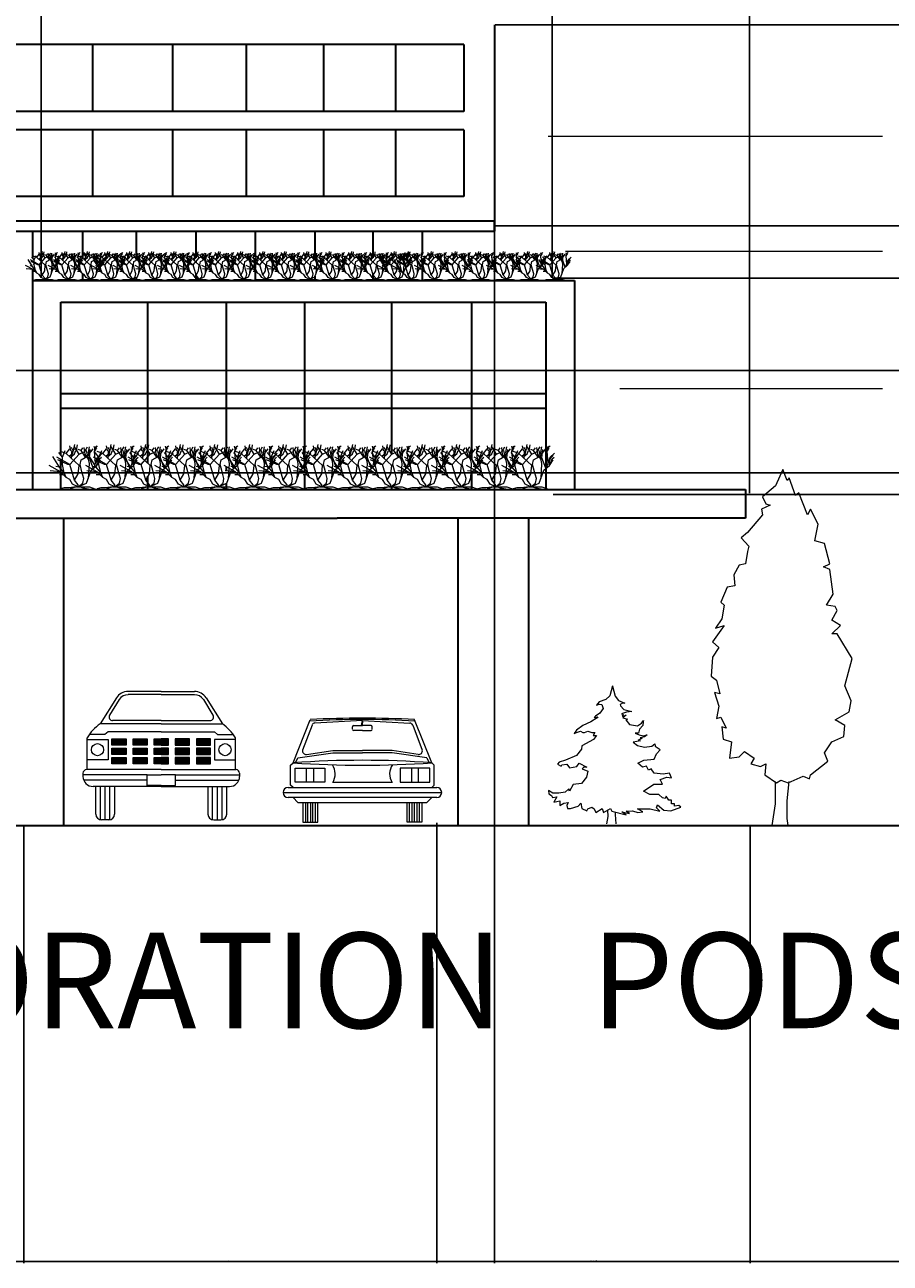
# Model space of a CAD drawing. Units: inches. Extents: x -160 to 434, y -145 to 103.
# Tile 5 of 7: x 176 to 262, y -145 to -22. Entities that reach past the tile are written whole.
import ezdxf

# ---------------------------------------------------------------- set-up
doc = ezdxf.new("R2010")
doc.units = ezdxf.units.IN
doc.header["$MEASUREMENT"] = 0
for name, color, linetype, lineweight in [('A-ANNO-DIMS', 2, 'Continuous', 18), ('A-ANNO-SYMB', 2, 'Continuous', 13), ('A-ANNO-TEXT', 3, 'Continuous', 18), ('A-ELEV', 7, 'Continuous', 35), ('A-ENTO-VEHC', 8, 'Continuous', 13), ('L-PLNT', 3, 'Continuous', 13)]:
    doc.layers.add(name, color=color, linetype=linetype, lineweight=lineweight)
doc.styles.get("Standard").update_dxf_attribs({"font": 'arial.ttf'})
doc.dimstyles.get("Standard").update_dxf_attribs({"dimtxt": 0.18, "dimasz": 0.18, "dimexe": 0.18, "dimexo": 0.0625, "dimgap": 0.09, "dimtad": 0, "dimtih": 1, "dimtoh": 1, "dimdec": 4, "dimzin": 0, "dimdsep": 46, "dimtxsty": 'Standard', "dimcen": 0.09, "dimadec": 0, "dimazin": 0, "dimtfac": 1, "dimtdec": 4, "dimtofl": 0, "dimtmove": 0, "dimatfit": 3, "dimfxl": 1, "dimtolj": 1, "dimtzin": 0, "dimarcsym": 0})

# ---------------------------------------------------------------- blocks, each defined once
blk = doc.blocks.new('*U2')
blk.add_lwpolyline([(-2.754, 191.699), (-6.78, 182.851), (-13.682, 176.953), (-11.956, 173.266), (-9.656, 172.529), (-14.257, 170.317), (-13.682, 167.368), (-21.733, 157.783), (-25.184, 154.834), (-21.158, 150.41), (-21.733, 147.461), (-22.884, 140.825), (-26.334, 140.087), (-29.21, 134.926), (-28.635, 129.028), (-32.661, 128.291), (-36.111, 120.18), (-34.386, 118.706), (-35.536, 111.333), (-38.987, 106.171), (-34.386, 107.646), (-40.712, 98.798), (-37.261, 95.849), (-40.712, 90.688), (-41.287, 80.366), (-38.412, 78.154), (-36.686, 70.781), (-39.562, 71.518), (-37.261, 64.145), (-38.412, 57.509), (-36.111, 58.247), (-33.236, 52.348), (-35.536, 53.086), (-34.961, 46.45), (-30.36, 44.975), (-31.51, 36.128), (-26.334, 36.865), (-23.459, 39.814), (-18.283, 36.128), (-20.008, 33.178), (-14.832, 31.704), (-11.956, 33.178), (-12.531, 27.28), (-6.205, 22.856), (-3.905, 24.331), (0.121, 22.856), (8.173, 26.543), (11.624, 25.068), (12.199, 27.28), (21.4, 34.653), (19.675, 39.077), (23.701, 44.975), (30.027, 47.924), (30.602, 53.823), (25.426, 56.772), (32.903, 61.196), (34.053, 67.094), (30.602, 75.205), (34.628, 89.951), (26.576, 103.222), (23.701, 103.222), (28.302, 107.646), (23.701, 110.595), (26.576, 115.756), (25.426, 117.968), (20.825, 118.706), (24.276, 124.604), (22.551, 137.876), (19.1, 139.35), (22.551, 140.825), (19.675, 151.884), (14.499, 153.359), (16.224, 162.207), (12.199, 170.317), (10.473, 167.368), (5.872, 179.165), (4.147, 177.69), (0.696, 187.275), (-0.454, 185.8)], close=True)
for points in [[(-6.813, 23.669), (-6.813, 11.669), (-8.627, 0)], [(0.387, 23.669), (-0.576, 13.271), (-0.576, 3.686), (0, 0)]]:
    blk.add_lwpolyline(points)
blk = doc.blocks.new('*U10')
for p, q in [((0, 69.27), (-17.87, 69.27)), ((0, 67.49), (-17.87, 67.49)), ((0, 69.27), (17.87, 69.27)), ((0, 67.49), (17.87, 67.49)), ((-24.18, 65.77), (-32.91, 51.76)), ((-22.67, 64.82), (-27.86, 56.49)), ((22.67, 64.82), (27.86, 56.49)), ((24.18, 65.77), (32.91, 51.76)), ((0, 53.54), (-26.22, 53.54)), ((0, 53.54), (26.22, 53.54)), ((0, 51.76), (-32.91, 51.76)), ((-28.59, 47.44), (-30.37, 45.96)), ((0, 47.44), (-28.59, 47.44)), ((0, 51.76), (32.91, 51.76)), ((0, 47.44), (28.59, 47.44)), ((28.59, 47.44), (30.37, 45.96)), ((-40.01, 27.08), (-40.01, 44.29)), ((-40.01, 43.31), (-28.69, 43.31)), ((-30.37, 45.96), (-38.87, 45.96)), ((-28.69, 43.31), (-28.69, 32.39)), ((-26.57, 40.26), (-26.57, 43.7)), ((-26.57, 43.7), (-18.89, 43.7)), ((-18.89, 40.26), (-26.57, 40.26)), ((-18.89, 43.7), (-18.89, 40.26)), ((-15.2, 43.7), (-7.53, 43.7)), ((-15.2, 40.26), (-15.2, 43.7)), ((-7.53, 40.26), (-15.2, 40.26)), ((-7.53, 43.7), (-7.53, 40.26)), ((-3.84, 40.26), (-3.84, 43.7)), ((-3.84, 43.7), (0, 43.7)), ((0, 40.26), (-3.84, 40.26)), ((3.84, 43.7), (0, 43.7)), ((0, 40.26), (3.84, 40.26)), ((3.84, 40.26), (3.84, 43.7)), ((7.53, 43.7), (7.53, 40.26)), ((15.2, 43.7), (7.53, 43.7)), ((7.53, 40.26), (15.2, 40.26)), ((15.2, 40.26), (15.2, 43.7)), ((26.57, 43.7), (18.89, 43.7)), ((18.89, 43.7), (18.89, 40.26)), ((18.89, 40.26), (26.57, 40.26)), ((26.57, 40.26), (26.57, 43.7)), ((28.69, 43.31), (28.69, 32.39)), ((40.01, 43.31), (28.69, 43.31)), ((30.37, 45.96), (38.87, 45.96)), ((40.01, 27.08), (40.01, 44.29)), ((-26.57, 35.24), (-26.57, 38.69)), ((-26.57, 38.69), (-18.89, 38.69)), ((-18.89, 35.24), (-26.57, 35.24)), ((-26.57, 30.23), (-26.57, 33.67)), ((-26.57, 33.67), (-18.89, 33.67)), ((-18.89, 38.69), (-18.89, 35.24)), ((-18.89, 33.67), (-18.89, 30.23)), ((-15.2, 38.69), (-7.53, 38.69)), ((-15.2, 35.24), (-15.2, 38.69)), ((-7.53, 35.24), (-15.2, 35.24)), ((-15.2, 33.67), (-7.53, 33.67)), ((-15.2, 30.23), (-15.2, 33.67)), ((-7.53, 38.69), (-7.53, 35.24)), ((-7.53, 33.67), (-7.53, 30.23)), ((-3.84, 35.24), (-3.84, 38.69)), ((-3.84, 38.69), (0, 38.69)), ((0, 35.24), (-3.84, 35.24)), ((-3.84, 30.23), (-3.84, 33.67)), ((-3.84, 33.67), (0, 33.67)), ((3.84, 38.69), (0, 38.69)), ((0, 35.24), (3.84, 35.24)), ((3.84, 33.67), (0, 33.67)), ((3.84, 35.24), (3.84, 38.69)), ((3.84, 30.23), (3.84, 33.67)), ((7.53, 38.69), (7.53, 35.24)), ((15.2, 38.69), (7.53, 38.69)), ((7.53, 35.24), (15.2, 35.24)), ((7.53, 33.67), (7.53, 30.23)), ((15.2, 33.67), (7.53, 33.67)), ((15.2, 35.24), (15.2, 38.69)), ((15.2, 30.23), (15.2, 33.67)), ((26.57, 38.69), (18.89, 38.69)), ((18.89, 38.69), (18.89, 35.24)), ((18.89, 35.24), (26.57, 35.24)), ((26.57, 33.67), (18.89, 33.67)), ((18.89, 33.67), (18.89, 30.23)), ((26.57, 35.24), (26.57, 38.69)), ((26.57, 30.23), (26.57, 33.67)), ((0, 27.08), (-40.3, 27.08)), ((-28.69, 32.39), (-40.01, 32.39)), ((-18.89, 30.23), (-26.57, 30.23)), ((-7.53, 30.23), (-15.2, 30.23)), ((0, 30.23), (-3.84, 30.23)), ((0, 30.23), (3.84, 30.23)), ((0, 27.08), (40.3, 27.08)), ((7.53, 30.23), (15.2, 30.23)), ((18.89, 30.23), (26.57, 30.23)), ((28.69, 32.39), (40.01, 32.39)), ((-42.18, 25.2), (-42.18, 23.46)), ((-7.63, 24.32), (-42.18, 24.32)), ((-7.63, 21.37), (-41.76, 21.37)), ((-7.63, 18.62), (-7.63, 24.32)), ((-7.63, 24.32), (0, 24.32)), ((7.63, 24.32), (0, 24.32)), ((7.63, 24.32), (42.18, 24.32)), ((7.63, 18.62), (7.63, 24.32)), ((7.63, 21.37), (41.76, 21.37)), ((42.18, 25.2), (42.18, 23.46)), ((0, 18.03), (-36.75, 18.03)), ((-35.26, 3.13), (-35.26, 18.03)), ((-32.73, 0.06), (-32.73, 18.03)), ((-30.2, 0), (-30.2, 18.03)), ((-27.66, 0.06), (-27.66, 18.03)), ((-25.13, 18.03), (-25.13, 3.13)), ((0, 18.62), (-7.63, 18.62)), ((0, 18.62), (7.63, 18.62)), ((0, 18.03), (36.75, 18.03)), ((25.13, 18.03), (25.13, 3.13)), ((27.66, 0.06), (27.66, 18.03)), ((30.2, 0), (30.2, 18.03)), ((32.73, 0.06), (32.73, 18.03)), ((35.26, 3.13), (35.26, 18.03)), ((-28.26, 0), (-32.13, 0)), ((28.26, 0), (32.13, 0))]:
    blk.add_line(p, q)
for centre in [(-34.35, 37.85), (34.35, 37.85)]:
    blk.add_circle(centre, 3.27)
for centre, radius, start, end in [((-17.87, 61.83), 7.44, 90, 148.09213), ((-17.87, 61.83), 5.65, 90, 148.09213), ((17.87, 61.83), 7.44, 31.90786, 90), ((17.87, 61.83), 5.65, 31.90786, 90), ((-26.22, 55.47), 1.92, 148.09213, 270), ((26.22, 55.47), 1.92, 270, 31.90786), ((-18.03, 30.48), 25.96, 124.96933, 147.86524), ((18.03, 30.48), 25.96, 32.13477, 55.03066), ((-40.3, 25.2), 1.88, 90, 180.00001), ((40.3, 25.2), 1.88, 0, 90), ((-36.75, 23.46), 5.43, 180.00001, 270), ((36.75, 23.46), 5.43, 270, 0), ((-32.13, 3.13), 3.13, 180.00001, 270), ((-28.26, 3.13), 3.13, 270, 0), ((28.26, 3.13), 3.13, 180.00001, 270), ((32.13, 3.13), 3.13, 270, 0)]:
    blk.add_arc(centre, radius, start, end)
for points in [[(-18.89, 43.7), (-18.89, 40.26), (-26.57, 43.7), (-26.57, 40.26)], [(-7.53, 43.7), (-7.53, 40.26), (-15.2, 43.7), (-15.2, 40.26)], [(0, 43.7), (0, 40.26), (-3.84, 43.7), (-3.84, 40.26)], [(0, 43.7), (0, 40.26), (3.84, 43.7), (3.84, 40.26)], [(7.53, 43.7), (7.53, 40.26), (15.2, 43.7), (15.2, 40.26)], [(18.89, 43.7), (18.89, 40.26), (26.57, 43.7), (26.57, 40.26)], [(-18.89, 38.69), (-18.89, 35.24), (-26.57, 38.69), (-26.57, 35.24)], [(-18.89, 33.67), (-18.89, 30.23), (-26.57, 33.67), (-26.57, 30.23)], [(-7.53, 38.69), (-7.53, 35.24), (-15.2, 38.69), (-15.2, 35.24)], [(-7.53, 33.67), (-7.53, 30.23), (-15.2, 33.67), (-15.2, 30.23)], [(0, 38.69), (0, 35.24), (-3.84, 38.69), (-3.84, 35.24)], [(0, 33.67), (0, 30.23), (-3.84, 33.67), (-3.84, 30.23)], [(0, 38.69), (0, 35.24), (3.84, 38.69), (3.84, 35.24)], [(0, 33.67), (0, 30.23), (3.84, 33.67), (3.84, 30.23)], [(7.53, 38.69), (7.53, 35.24), (15.2, 38.69), (15.2, 35.24)], [(7.53, 33.67), (7.53, 30.23), (15.2, 33.67), (15.2, 30.23)], [(18.89, 38.69), (18.89, 35.24), (26.57, 38.69), (26.57, 35.24)], [(18.89, 33.67), (18.89, 30.23), (26.57, 33.67), (26.57, 30.23)]]:
    blk.add_solid(points)
blk = doc.blocks.new('*U11')
for p, q in [((-37.38, 32.04), (-28.11, 55.23)), ((-0.21, 54.74), (-0.67, 52.07)), ((0.21, 54.74), (-0.23, 52.08)), ((37.38, 32.04), (28.11, 55.23)), ((-36.05, 32.04), (-34.71, 34.71)), ((-34.71, 34.71), (-16.02, 37.38)), ((-16.02, 37.38), (0, 37.38)), ((16.02, 37.38), (0, 37.38)), ((34.71, 34.71), (16.02, 37.38)), ((34.71, 34.71), (36.05, 32.04)), ((-38.72, 30.71), (-37.38, 32.04)), ((-38.72, 20.03), (-38.72, 30.71)), ((38.72, 30.71), (37.38, 32.04)), ((38.72, 20.03), (38.72, 30.71)), ((-37.38, 18.69), (-38.72, 20.03)), ((16.02, 21.36), (-16.02, 21.36)), ((37.38, 18.69), (38.72, 20.03)), ((-42.72, 16.02), (42.72, 16.02)), ((-40.05, 18.69), (40.05, 18.69)), ((40.05, 13.35), (-40.05, 13.35)), ((-37.38, 13.35), (-34.71, 10.68)), ((34.71, 10.68), (37.38, 13.35)), ((-34.71, 10.68), (34.71, 10.68)), ((-32.04, 10.68), (-32.04, 0)), ((-30.71, 10.68), (-30.71, 0)), ((-29.37, 0), (-29.37, 10.68)), ((-28.04, 10.68), (-28.04, 0)), ((-26.7, 0), (-26.7, 10.68)), ((-25.37, 10.68), (-25.37, 0)), ((-24.03, 0), (-24.03, 10.68)), ((24.03, 0), (24.03, 10.68)), ((25.37, 0), (25.37, 10.68)), ((26.7, 10.68), (26.7, 0)), ((28.04, 0), (28.04, 10.68)), ((29.37, 10.68), (29.37, 0)), ((30.71, 0), (30.71, 10.68)), ((32.04, 10.68), (32.04, 0)), ((-32.04, 0), (-24.03, 0)), ((32.04, 0), (24.03, 0))]:
    blk.add_line(p, q)
for points in [[(0, 54.74), (-25.63, 53.46)], [(0.01, 54.74), (25.64, 53.45)], [(-27.12, 52.31), (-32.28, 38.89)], [(-5.34, 50.07), (-5.34, 51.4)], [(-4.67, 52.07), (0, 52.07)], [(0, 49.4), (-4.67, 49.4)], [(4.67, 52.07), (0, 52.07)], [(0, 49.4), (4.67, 49.4)], [(5.34, 50.07), (5.34, 51.4)], [(27.13, 52.3), (32.28, 38.88)], [(-30.06, 36.56), (-16.02, 38.72), (0, 38.72)], [(30.06, 36.54), (16.02, 38.71), (0, 38.72)]]:
    blk.add_lwpolyline(points)
for points in [[(-36.27, 29.17), (-20.26, 29.17), (-20.26, 21.57), (-36.27, 21.57)], [(-30.17, 29.17), (-26.37, 29.17), (-26.37, 21.57), (-30.17, 21.57)], [(36.27, 29.17), (20.26, 29.17), (20.26, 21.57), (36.27, 21.57)], [(30.17, 29.17), (26.37, 29.17), (26.37, 21.57), (30.17, 21.57)]]:
    blk.add_lwpolyline(points, close=True)
for centre, radius, start, end in [((0, -432), 487.32, 86.65721, 93.3419), ((0, -431.24), 487.32, 86.69396, 93.3033), ((-25.37, 51.59), 1.89, 97.4497, 154.9311), ((25.37, 51.57), 1.89, 25.04208, 82.52346), ((-4.67, 51.4), 0.668, 93.60832, 178.1081), ((-4.67, 50.07), 0.668, 184.4192, 266.4386), ((4.67, 51.4), 0.668, 1.89193, 86.39168), ((4.67, 50.07), 0.668, 273.5614, 355.5808), ((0, -490.66), 524.03, 85.90918, 94.09081), ((-30.43, 38.42), 1.89, 166.5724, 279.9572), ((30.43, 38.41), 1.89, 260.016, 13.40079), ((0, 554.74), 524.03, 265.90919, 274.09082), ((-23.36, 26.03), 8.7, 327.5288, 34.44428), ((23.36, 26.03), 8.7, 145.55569, 212.4712), ((-40.05, 16.02), 2.67, 90, 270), ((40.05, 16.02), 2.67, 270, 90)]:
    blk.add_arc(centre, radius, start, end)
blk = doc.blocks.new('*U5')
for p, q in [((-14.88, 18.24), (-17.76, 19.2)), ((-16.8, 16.32), (-15.36, 19.68)), ((-14.88, 18.24), (-12.96, 20.64)), ((-12.471, 19.775), (-12.898, 22.044)), ((-11.677, 19.071), (-12.471, 19.775)), ((-11.28, 19.619), (-12.104, 21.184)), ((-11.921, 18.836), (-10.64, 20.401)), ((-11.433, 18.289), (-10.457, 22.749)), ((-10.579, 18.054), (-9.846, 19.697)), ((-8.16, 17.76), (-10.56, 21.6)), ((-9.48, 19.775), (-8.992, 22.592)), ((-7.2, 19.68), (-8.64, 20.16)), ((-8.16, 17.76), (-5.28, 19.2)), ((-7.2, 19.68), (-6.24, 21.12)), ((-4.8, 16.32), (-7.2, 19.68)), ((-5.086, 17.741), (-5.513, 21.34)), ((-5.28, 19.2), (-3.84, 21.6)), ((-2.88, 12.96), (-4.32, 19.68)), ((-3.84, 16.8), (-0.96, 20.64)), ((-3.377, 18.602), (-2.888, 21.575)), ((-2.88, 15.84), (-2.4, 20.16)), ((-0.508, 21.888), (-0.081, 20.558)), ((-0.203, 19.149), (0.102, 21.34)), ((-0.142, 19.384), (0.59, 20.401)), ((-0.02, 20.01), (0.896, 21.105)), ((0.041, 20.714), (1.384, 22.044)), ((0.102, 21.34), (0.835, 21.888)), ((-18.24, 11.04), (-21.755, 16.655)), ((-12.96, 12.48), (-19.68, 16.32)), ((-13.92, 12.48), (-19.2, 14.88)), ((-16.8, 16.32), (-18.72, 18.72)), ((-16.8, 12.48), (-17.76, 12.96)), ((-16.8, 12.48), (-16.8, 16.32)), ((-8.16, 12), (-14.88, 18.24)), ((-13.325, 16.724), (-11.433, 18.289)), ((-12.96, 12.48), (-8.16, 17.76)), ((-12.043, 15.628), (-11.921, 18.836)), ((-11.982, 16.802), (-10.579, 18.054)), ((-7.68, 12.48), (-7.2, 14.88)), ((-7.2, 14.88), (-3.84, 16.8)), ((-3.377, 15.315), (-5.086, 17.819)), ((-2.766, 16.802), (-3.377, 18.602)), ((-3.36, 5.28), (-2.88, 12.96)), ((-0.96, 10.56), (-2.88, 15.84)), ((-0.48, 10.8), (0.346, 13.203)), ((0.346, 13.203), (-0.203, 19.149)), ((0.346, 13.203), (1.323, 16.254)), ((0.96, 12), (1.44, 15.36)), ((0.96, 12), (2.88, 14.88)), ((1.323, 16.254), (3.642, 18.289)), ((1.44, 15.36), (2.88, 17.28)), ((1.92, 13.44), (2.4, 15.36)), ((2.4, 15.36), (3.36, 16.32)), ((-17.76, 8.64), (-23.663, 11.961)), ((-17.76, 8.64), (-23.128, 9.222)), ((-18.24, 11.04), (-20.16, 11.52)), ((-15.84, 8.16), (-18.24, 11.04)), ((-16.32, 7.2), (-18.24, 7.2)), ((-14.88, 5.76), (-17.76, 8.64)), ((-15.84, 8.16), (-16.8, 12.48)), ((-14.88, 5.76), (-15.84, 8.16)), ((-12.96, 12.48), (-13.92, 12.48)), ((-10.56, 4.32), (-12.96, 12.48)), ((-10.56, 4.32), (-8.64, 7.68)), ((-8.64, 7.68), (-8.16, 12)), ((-6.72, 8.64), (-7.68, 12.48)), ((-5.76, 5.28), (-6.72, 8.64)), ((-4.32, 2.88), (-1.92, 9.6)), ((-1.92, 9.6), (0.96, 12)), ((-15.84, 0.48), (-17.76, 0)), ((-13.44, 0.48), (-15.84, 0.48)), ((-12.96, 4.8), (-14.88, 5.76)), ((-9.6, 0.96), (-13.44, 0.48)), ((-11.52, 2.4), (-12.96, 4.8)), ((-9.6, 0.96), (-12.96, 0)), ((-8.64, 0.96), (-11.52, 2.4)), ((-8.64, 1.92), (-10.56, 4.32)), ((-9.6, 0.96), (-7.68, 0.96)), ((-8.64, 0.96), (-4.32, 2.88)), ((-8.64, 0.96), (-6.24, 2.88)), ((-8.64, 0.96), (-8.64, 1.92)), ((-8.64, 0.96), (-2.88, 0.96)), ((-7.68, 0.96), (-6.24, 0.48)), ((-6.24, 2.88), (-5.76, 5.28)), ((-6.24, 0.48), (-3.36, 0)), ((-2.88, 0.96), (0, 0))]:
    blk.add_line(p, q)
blk = doc.blocks.new('*U7')
for p, q in [((-8.263, 7.598), (-8.747, 14.105)), ((-9.75, 0), (-8.263, 7.598)), ((-0.771, 9.56), (-0.69, 11.833)), ((0, 0), (-0.771, 9.56))]:
    blk.add_line(p, q)
for points in [[(-3.9, 142.35), (-6.596, 132.037), (-10.801, 128.443), (-17.81, 126.047), (-20.614, 122.452), (-17.81, 123.65), (-15.007, 123.051), (-13.605, 118.858), (-16.876, 114.065), (-21.549, 111.07), (-22.951, 109.872), (-19.212, 110.471), (-19.68, 109.273), (-26.222, 105.079), (-34.633, 101.485), (-41.175, 96.693), (-43.511, 93.098), (-41.175, 94.296), (-36.969, 95.494), (-34.633, 94.296), (-32.764, 94.296), (-29.493, 95.494)], [(-3.759, 141.97), (-1.074, 131.643), (2.437, 127.141), (8.84, 124.493), (6.568, 124.493), (4.09, 123.169), (4.296, 121.846), (7.807, 117.874), (16.069, 116.02), (10.492, 115.226), (5.535, 113.372), (6.981, 112.843), (5.948, 110.989), (10.286, 112.048), (6.775, 109.401), (11.732, 108.077), (9.873, 107.282), (13.797, 102.516), (21.852, 101.192), (25.983, 103.84), (28.048, 106.488), (27.842, 105.164), (27.429, 101.457), (24.124, 97.75), (23.091, 93.513), (19.58, 93.513), (23.505, 91.66), (28.255, 90.866), (31.973, 91.925), (29.081, 89.806), (24.537, 88.747), (26.809, 88.218), (22.472, 86.099), (24.95, 85.57), (17.308, 84.246), (21.852, 80.804), (29.081, 79.215), (36.723, 80.009), (39.821, 82.392), (40.028, 80.009), (45.398, 76.567)], [(-29.25, 95.55), (-25.287, 94.296), (-22.016, 94.296), (-23.885, 91.301), (-20.614, 91.301), (-23.418, 87.108), (-35.567, 80.518), (-36.035, 76.924), (-41.175, 70.334), (-52.389, 65.542), (-58.931, 63.744), (-60.8, 61.348), (-57.062, 59.551), (-56.128, 60.749), (-50.987, 61.348), (-48.184, 57.754), (-40.707, 58.952), (-38.371, 62.546), (-30.427, 58.353), (-33.698, 58.353), (-35.1, 56.556), (-29.493, 54.159), (-30.894, 48.169), (-36.035, 41.579), (-44.446, 40.381), (-48.184, 33.791), (-49.118, 36.188), (-52.857, 32.593), (-59.399, 31.395), (-65.473, 31.395), (-70.146, 34.39), (-69.679, 30.796), (-66.875, 28.999), (-65.941, 27.202), (-61.268, 27.801), (-64.539, 22.409), (-58.464, 23.607), (-58.464, 18.815), (-54.258, 21.211), (-49.586, 21.81), (-50.987, 18.815), (-50.52, 15.82), (-47.249, 15.82), (-39.306, 18.216), (-36.502, 21.211), (-35.567, 15.82), (-30.427, 13.423), (-29.493, 15.221), (-25.287, 17.018), (-22.951, 15.221), (-21.081, 11.626), (-14.539, 15.82), (-13.138, 11.626), (-6.128, 15.82), (-4.726, 12.824), (10.226, 9.23), (5.554, 12.225), (13.497, 10.428), (10.226, 12.824), (16.768, 13.423), (22.376, 11.626), (27.516, 12.225), (21.909, 15.221), (34.993, 15.221), (44.806, 12.824), (41.535, 16.419), (42.469, 19.414), (49.011, 14.023), (56.487, 13.423), (66.768, 17.018), (64.431, 18.815), (60.226, 18.216), (60.226, 20.612), (56.955, 20.612), (56.955, 24.206), (54.151, 24.206), (51.348, 28.4), (50.413, 26.004), (47.609, 26.603), (43.871, 30.197), (38.731, 30.197), (34.525, 30.197), (27.983, 33.791), (38.731, 40.98), (47.609, 40.98), (45.273, 45.773), (52.282, 48.169), (56.955, 47.57), (55.086, 52.362), (48.544, 51.164), (39.198, 52.362), (35.927, 56.556), (33.123, 55.357), (31.254, 59.551), (27.049, 58.353), (22.376, 62.546), (28.451, 65.542), (39.198, 66.74), (41.535, 72.131), (45.273, 76.325)]]:
    blk.add_lwpolyline(points)
blk = doc.blocks.new('*D12')
at = {"layer": 'A-ANNO-DIMS', "color": 0, "lineweight": -2, "transparency": 16777216}
for p, q in [((-84.07, -101.41), (-84.07, -144.81)), ((403.75, -101.41), (403.75, -144.81)), ((-83.89, -144.63), (159.44, -144.63)), ((403.57, -144.63), (160.24, -144.63))]:
    blk.add_line(p, q, dxfattribs=at)
at = {"layer": 'A-ANNO-DIMS', "color": 0, "transparency": 16777216}
for points in [[(-83.89, -144.6), (-83.89, -144.66), (-84.07, -144.63)], [(403.57, -144.6), (403.57, -144.66), (403.75, -144.63)]]:
    blk.add_solid(points, dxfattribs=at)
at = {"layer": 'Defpoints', "color": 0, "transparency": 16777216}
for p in [(-84.07, -101.35), (403.75, -101.35), (403.75, -144.63)]:
    blk.add_point(p, dxfattribs=at)
at = {"layer": 'A-ANNO-DIMS', "color": 0, "transparency": 16777216, "insert": (159.84, -144.63), "char_height": 0.18, "attachment_point": 5}
blk.add_mtext('\\A1;487.8', dxfattribs=at)
blk = doc.blocks.new('*D22')
at = {"layer": 'A-ANNO-DIMS', "color": 0, "lineweight": -2, "transparency": 16777216}
for p, q in [((175.81, -101.41), (175.81, -144.81)), ((216.81, -101.09), (216.81, -144.81)), ((175.99, -144.63), (195.91, -144.63)), ((216.63, -144.63), (196.71, -144.63))]:
    blk.add_line(p, q, dxfattribs=at)
at = {"layer": 'A-ANNO-DIMS', "color": 0, "transparency": 16777216}
for points in [[(175.99, -144.6), (175.99, -144.66), (175.81, -144.63)], [(216.63, -144.6), (216.63, -144.66), (216.81, -144.63)]]:
    blk.add_solid(points, dxfattribs=at)
at = {"layer": 'Defpoints', "color": 0, "transparency": 16777216}
for p in [(175.81, -101.35), (216.81, -101.02), (216.81, -144.63)]:
    blk.add_point(p, dxfattribs=at)
at = {"layer": 'A-ANNO-DIMS', "color": 0, "transparency": 16777216, "insert": (196.31, -144.63), "char_height": 0.18, "attachment_point": 5}
blk.add_mtext('\\A1;40.99', dxfattribs=at)
blk = doc.blocks.new('*D23')
at = {"layer": 'A-ANNO-DIMS', "color": 0, "lineweight": -2, "transparency": 16777216}
for p, q in [((216.81, -101.09), (216.81, -144.81)), ((247.94, -101.38), (247.94, -144.81)), ((216.99, -144.63), (231.91, -144.63)), ((247.76, -144.63), (232.84, -144.63))]:
    blk.add_line(p, q, dxfattribs=at)
at = {"layer": 'A-ANNO-DIMS', "color": 0, "transparency": 16777216}
for points in [[(216.99, -144.6), (216.99, -144.66), (216.81, -144.63)], [(247.76, -144.6), (247.76, -144.66), (247.94, -144.63)]]:
    blk.add_solid(points, dxfattribs=at)
at = {"layer": 'Defpoints', "color": 0, "transparency": 16777216}
for p in [(216.81, -101.02), (247.94, -101.32), (247.94, -144.63)]:
    blk.add_point(p, dxfattribs=at)
at = {"layer": 'A-ANNO-DIMS', "color": 0, "transparency": 16777216, "insert": (232.37, -144.63), "char_height": 0.18, "attachment_point": 5}
blk.add_mtext('\\A1;31.135', dxfattribs=at)
blk = doc.blocks.new('*D31')
at = {"layer": 'A-ANNO-DIMS', "color": 0, "lineweight": -2, "transparency": 16777216}
for p, q in [((107.33, 8.95), (433.98, 8.95)), ((433.8, 8.77), (433.8, -23.43)), ((433.8, -55.99), (433.8, -23.79)), ((107.33, -56.17), (433.98, -56.17))]:
    blk.add_line(p, q, dxfattribs=at)
at = {"layer": 'A-ANNO-DIMS', "color": 0, "transparency": 16777216}
for points in [[(433.77, 8.77), (433.83, 8.77), (433.8, 8.95)], [(433.77, -55.99), (433.83, -55.99), (433.8, -56.17)]]:
    blk.add_solid(points, dxfattribs=at)
at = {"layer": 'Defpoints', "color": 0, "transparency": 16777216}
for p in [(107.27, 8.95), (107.27, -56.17), (433.8, -56.17)]:
    blk.add_point(p, dxfattribs=at)
at = {"layer": 'A-ANNO-DIMS', "color": 0, "transparency": 16777216, "insert": (433.8, -23.61), "char_height": 0.18, "attachment_point": 5}
blk.add_mtext('\\A1;65.11', dxfattribs=at)
blk = doc.blocks.new('*D32')
at = {"layer": 'A-ANNO-DIMS', "color": 0, "lineweight": -2, "transparency": 16777216}
for p, q in [((107.33, -56.17), (433.98, -56.17)), ((433.8, -56.35), (433.8, -61.07)), ((433.8, -66.15), (433.8, -61.43)), ((106.73, -66.33), (433.98, -66.33))]:
    blk.add_line(p, q, dxfattribs=at)
at = {"layer": 'A-ANNO-DIMS', "color": 0, "transparency": 16777216}
for points in [[(433.77, -56.35), (433.83, -56.35), (433.8, -56.17)], [(433.77, -66.15), (433.83, -66.15), (433.8, -66.33)]]:
    blk.add_solid(points, dxfattribs=at)
at = {"layer": 'Defpoints', "color": 0, "transparency": 16777216}
for p in [(107.27, -56.17), (106.67, -66.33), (433.8, -66.33)]:
    blk.add_point(p, dxfattribs=at)
at = {"layer": 'A-ANNO-DIMS', "color": 0, "transparency": 16777216, "insert": (433.8, -61.25), "char_height": 0.18, "attachment_point": 5}
blk.add_mtext('\\A1;10.165', dxfattribs=at)
blk = doc.blocks.new('*D41')
at = {"layer": 'A-ANNO-DIMS', "color": 0, "lineweight": -2, "transparency": 16777216}
for p, q in [((124.65, -41.4), (124.65, -144.81)), ((222.55, -41.85), (222.55, -144.81)), ((124.83, -144.63), (173.28, -144.63)), ((222.37, -144.63), (173.93, -144.63))]:
    blk.add_line(p, q, dxfattribs=at)
at = {"layer": 'A-ANNO-DIMS', "color": 0, "transparency": 16777216}
for points in [[(124.83, -144.6), (124.83, -144.66), (124.65, -144.63)], [(222.37, -144.6), (222.37, -144.66), (222.55, -144.63)]]:
    blk.add_solid(points, dxfattribs=at)
at = {"layer": 'Defpoints', "color": 0, "transparency": 16777216}
for p in [(124.65, -41.34), (222.55, -41.79), (222.55, -144.63)]:
    blk.add_point(p, dxfattribs=at)
at = {"layer": 'A-ANNO-DIMS', "color": 0, "transparency": 16777216, "insert": (173.6, -144.63), "char_height": 0.18, "attachment_point": 5}
blk.add_mtext('\\A1;97.9', dxfattribs=at)
blk = doc.blocks.new('*D42')
at = {"layer": 'A-ANNO-DIMS', "color": 0, "lineweight": -2, "transparency": 16777216}
for p, q in [((222.59, -21.84), (433.98, -21.84)), ((433.8, -22.02), (433.8, -31.63)), ((433.8, -41.61), (433.8, -31.99)), ((222.62, -41.79), (433.98, -41.79))]:
    blk.add_line(p, q, dxfattribs=at)
at = {"layer": 'A-ANNO-DIMS', "color": 0, "transparency": 16777216}
for points in [[(433.77, -22.02), (433.83, -22.02), (433.8, -21.84)], [(433.77, -41.61), (433.83, -41.61), (433.8, -41.79)]]:
    blk.add_solid(points, dxfattribs=at)
at = {"layer": 'Defpoints', "color": 0, "transparency": 16777216}
for p in [(222.53, -21.84), (222.55, -41.79), (433.8, -41.79)]:
    blk.add_point(p, dxfattribs=at)
at = {"layer": 'A-ANNO-DIMS', "color": 0, "transparency": 16777216, "insert": (433.8, -31.81), "char_height": 0.18, "attachment_point": 5}
blk.add_mtext('\\A1;19.946', dxfattribs=at)
blk = doc.blocks.new('*D43')
at = {"layer": 'A-ANNO-DIMS', "color": 0, "lineweight": -2, "transparency": 16777216}
for p, q in [((222.5, -5.64), (433.98, -5.64)), ((433.8, -5.82), (433.8, -13.56)), ((433.8, -21.66), (433.8, -13.92)), ((222.59, -21.84), (433.98, -21.84))]:
    blk.add_line(p, q, dxfattribs=at)
at = {"layer": 'A-ANNO-DIMS', "color": 0, "transparency": 16777216}
for points in [[(433.77, -5.82), (433.83, -5.82), (433.8, -5.64)], [(433.77, -21.66), (433.83, -21.66), (433.8, -21.84)]]:
    blk.add_solid(points, dxfattribs=at)
at = {"layer": 'Defpoints', "color": 0, "transparency": 16777216}
for p in [(222.44, -5.64), (222.53, -21.84), (433.8, -21.84)]:
    blk.add_point(p, dxfattribs=at)
at = {"layer": 'A-ANNO-DIMS', "color": 0, "transparency": 16777216, "insert": (433.8, -13.74), "char_height": 0.18, "attachment_point": 5}
blk.add_mtext('\\A1;16.204', dxfattribs=at)
blk = doc.blocks.new('*D44')
at = {"layer": 'A-ANNO-DIMS', "color": 0, "lineweight": -2, "transparency": 16777216}
for p, q in [((177.54, -46.95), (177.54, 102.5)), ((177.72, 102.32), (202.52, 102.32)), ((228.07, 102.32), (203.27, 102.32)), ((228.25, -46.95), (228.25, 102.5))]:
    blk.add_line(p, q, dxfattribs=at)
at = {"layer": 'A-ANNO-DIMS', "color": 0, "transparency": 16777216}
for points in [[(177.72, 102.35), (177.72, 102.29), (177.54, 102.32)], [(228.07, 102.35), (228.07, 102.29), (228.25, 102.32)]]:
    blk.add_solid(points, dxfattribs=at)
at = {"layer": 'Defpoints', "color": 0, "transparency": 16777216}
for p in [(228.25, 102.32), (177.54, -47.01), (228.25, -47.01)]:
    blk.add_point(p, dxfattribs=at)
at = {"layer": 'A-ANNO-DIMS', "color": 0, "transparency": 16777216, "insert": (202.89, 102.32), "char_height": 0.18, "attachment_point": 5}
blk.add_mtext('\\A1;50.71', dxfattribs=at)
blk = doc.blocks.new('*D45')
at = {"layer": 'A-ANNO-DIMS', "color": 0, "lineweight": -2, "transparency": 16777216}
for p, q in [((228.31, -47.01), (433.98, -47.01)), ((433.8, -47.19), (433.8, -57.57)), ((433.8, -68.3), (433.8, -57.93)), ((228.35, -68.48), (433.98, -68.48))]:
    blk.add_line(p, q, dxfattribs=at)
at = {"layer": 'A-ANNO-DIMS', "color": 0, "transparency": 16777216}
for points in [[(433.77, -47.19), (433.83, -47.19), (433.8, -47.01)], [(433.77, -68.3), (433.83, -68.3), (433.8, -68.48)]]:
    blk.add_solid(points, dxfattribs=at)
at = {"layer": 'Defpoints', "color": 0, "transparency": 16777216}
for p in [(228.25, -47.01), (228.29, -68.48), (433.8, -68.48)]:
    blk.add_point(p, dxfattribs=at)
at = {"layer": 'A-ANNO-DIMS', "color": 0, "transparency": 16777216, "insert": (433.8, -57.75), "char_height": 0.18, "attachment_point": 5}
blk.add_mtext('\\A1;21.473', dxfattribs=at)
blk = doc.blocks.new('*D46')
at = {"layer": 'A-ANNO-DIMS', "color": 0, "lineweight": -2, "transparency": 16777216}
for p, q in [((222.62, -41.79), (433.98, -41.79)), ((433.8, -41.97), (433.8, -54.95)), ((433.8, -68.3), (433.8, -55.32)), ((228.35, -68.48), (433.98, -68.48))]:
    blk.add_line(p, q, dxfattribs=at)
at = {"layer": 'A-ANNO-DIMS', "color": 0, "transparency": 16777216}
for points in [[(433.77, -41.97), (433.83, -41.97), (433.8, -41.79)], [(433.77, -68.3), (433.83, -68.3), (433.8, -68.48)]]:
    blk.add_solid(points, dxfattribs=at)
at = {"layer": 'Defpoints', "color": 0, "transparency": 16777216}
for p in [(222.55, -41.79), (228.29, -68.48), (433.8, -68.48)]:
    blk.add_point(p, dxfattribs=at)
at = {"layer": 'A-ANNO-DIMS', "color": 0, "transparency": 16777216, "insert": (433.8, -55.14), "char_height": 0.18, "attachment_point": 5}
blk.add_mtext('\\A1;26.7', dxfattribs=at)
blk = doc.blocks.new('*D48')
at = {"layer": 'A-ANNO-DIMS', "color": 0, "lineweight": -2, "transparency": 16777216}
for p, q in [((228.25, -46.95), (228.25, 102.5)), ((228.43, 102.32), (237.61, 102.32)), ((247.69, 102.32), (238.52, 102.32)), ((247.87, -68.35), (247.87, 102.5))]:
    blk.add_line(p, q, dxfattribs=at)
at = {"layer": 'A-ANNO-DIMS', "color": 0, "transparency": 16777216}
for points in [[(228.43, 102.35), (228.43, 102.29), (228.25, 102.32)], [(247.69, 102.35), (247.69, 102.29), (247.87, 102.32)]]:
    blk.add_solid(points, dxfattribs=at)
at = {"layer": 'Defpoints', "color": 0, "transparency": 16777216}
for p in [(247.87, 102.32), (228.25, -47.01), (247.87, -68.41)]:
    blk.add_point(p, dxfattribs=at)
at = {"layer": 'A-ANNO-DIMS', "color": 0, "transparency": 16777216, "insert": (238.06, 102.32), "char_height": 0.18, "attachment_point": 5}
blk.add_mtext('\\A1;19.626', dxfattribs=at)

msp = doc.modelspace()

# ---------------------------------------------------------------- linework, layer by layer
at = {"layer": 'A-ANNO-SYMB'}
for p, q in [((227.8844, -32.9114), (261.0586, -32.9114)), ((229.5882, -44.311), (261.0586, -44.311)), ((234.9964, -57.9615), (261.0586, -57.9615))]:
    msp.add_line(p, q, dxfattribs=at)
at = {"layer": 'A-ELEV'}
for p, q in [((222.5284, -21.8399), (222.5284, -41.3403)), ((219.5071, -23.7966), (137.8943, -23.7966)), ((182.6363, -23.7966), (182.6363, -30.4469)), ((190.5577, -23.7966), (190.5577, -30.4469)), ((197.8904, -23.7966), (197.8904, -30.4469)), ((205.5441, -23.7966), (205.5441, -30.4469)), ((212.7162, -23.7966), (212.7162, -30.4469)), ((219.5071, -23.7966), (219.5071, -30.4469)), ((219.5071, -30.4469), (137.8943, -30.4469)), ((219.5071, -32.2746), (137.8943, -32.2746)), ((182.6363, -32.2746), (182.6363, -38.9063)), ((190.5577, -32.2746), (190.5577, -38.9063)), ((197.8904, -32.2746), (197.8904, -38.9063)), ((205.5441, -32.2746), (205.5441, -38.9063)), ((212.7162, -32.2746), (212.7162, -38.9063)), ((219.5071, -32.2746), (219.5071, -38.9063)), ((219.5071, -38.9063), (137.8943, -38.9063)), ((213.3013, -41.3403), (137.8943, -41.3403)), ((222.5284, -41.3403), (213.3013, -41.3403)), ((222.5284, -42.3312), (222.5284, -41.3403)), ((222.5284, -41.3403), (222.5284, -42.3312)), ((134.424, -42.3312), (222.5284, -42.3312)), ((176.7032, -45.0029), (176.7032, -42.3312)), ((181.6669, -45.0298), (181.6669, -42.3312)), ((187.0005, -45.2101), (187.0005, -42.3312)), ((192.9108, -44.9671), (192.9108, -42.3312)), ((198.821, -44.8774), (198.821, -42.3312)), ((204.7313, -45.1679), (204.7313, -42.3312)), ((210.4974, -44.9666), (210.4974, -42.3312)), ((215.3986, -44.599), (215.3986, -42.3312)), ((176.7032, -45.4341), (176.7032, -45.306)), ((192.9108, -45.4327), (192.9108, -45.3417)), ((198.821, -45.2374), (198.821, -45.025)), ((198.821, -45.9595), (198.821, -45.4239)), ((210.4974, -45.4332), (210.4974, -45.3411)), ((215.3986, -47.2473), (215.3986, -45.4187)), ((176.7032, -67.9742), (176.7032, -46.137)), ((181.6669, -45.654), (181.6669, -45.5823)), ((181.6669, -47.2473), (181.6669, -46.5617)), ((192.9108, -47.2473), (192.9108, -46.6571)), ((198.821, -47.2473), (198.821, -46.1421)), ((204.7313, -46.0946), (204.7313, -45.8713)), ((210.4974, -47.2473), (210.4974, -46.659)), ((176.7032, -47.2473), (230.4935, -47.2473)), ((187.0005, -47.2473), (187.0005, -46.9196)), ((204.7313, -47.2473), (204.7313, -46.8045)), ((230.4935, -47.2473), (230.4935, -67.9742)), ((179.4767, -49.3965), (227.6491, -49.3965)), ((179.4767, -64.5686), (179.4767, -49.3965)), ((188.1294, -65.3772), (188.1294, -49.3965)), ((195.9136, -64.7492), (195.9136, -49.3965)), ((203.6979, -66.3113), (203.6979, -49.3965)), ((212.3471, -64.4939), (212.3471, -49.3965)), ((220.2755, -64.9339), (220.2755, -49.3965)), ((227.6491, -49.3965), (227.6491, -67.9742)), ((179.4767, -58.4673), (227.6491, -58.4673)), ((179.4767, -59.9071), (227.6491, -59.9071)), ((179.4767, -67.9742), (179.4767, -64.9915)), ((195.9136, -66.142), (195.9136, -65.7237)), ((212.3471, -65.6484), (212.3471, -65.59)), ((220.2755, -67.9742), (220.2755, -66.1744)), ((188.1294, -67.9742), (188.1294, -66.6764)), ((195.9136, -67.9742), (195.9136, -67.3688)), ((203.6979, -67.9742), (203.6979, -66.5188)), ((2.6577, -67.9742), (206.9244, -67.9742)), ((206.9244, -67.9742), (234.4392, -67.9742)), ((212.3471, -67.9742), (212.3471, -67.65)), ((234.4392, -67.9742), (247.4785, -67.9742)), ((247.4785, -67.9742), (247.4785, -70.8373)), ((2.6577, -70.8373), (206.9244, -70.8373)), ((179.7503, -70.8373), (179.7503, -101.346)), ((234.4392, -70.8373), (206.9244, -70.8373)), ((218.9112, -70.8373), (218.9112, -101.346)), ((225.9234, -70.8373), (225.9234, -101.346)), ((237.2836, -70.8373), (234.4392, -70.8373)), ((247.4785, -70.8373), (237.2836, -70.8373)), ((2.6577, -101.346), (403.7477, -101.346))]:
    msp.add_line(p, q, dxfattribs=at)

# ---------------------------------------------------------------- block references
at = {"layer": 'A-ENTO-VEHC', "xscale": 0.1843091790693797, "yscale": 0.1843091790693797, "zscale": 0.1843091790693797}
for name, p in [('*U10', (189.4517, -100.7948)), ('*U11', (209.4233, -101.0241))]:
    msp.add_blockref(name, p, dxfattribs=at)
at = {"layer": 'L-PLNT'}
for name, p, xscale, yscale, zscale in [('*U5', (178.9641, -47.2383), 0.1262102187894788, 0.1262102187894788, 0.1262102187894788), ('*U5', (181.2215, -47.2383), 0.1262102187894788, 0.1262102187894788, 0.1262102187894788), ('*U5', (183.4441, -47.2383), 0.1262102187894788, 0.1262102187894788, 0.1262102187894788), ('*U5', (185.4758, -47.2383), 0.1262102187894788, 0.1262102187894788, 0.1262102187894788), ('*U5', (187.6464, -47.2383), 0.1262102187894788, 0.1262102187894788, 0.1262102187894788), ('*U5', (189.8435, -47.2383), 0.1262102187894788, 0.1262102187894788, 0.1262102187894788), ('*U5', (192.0662, -47.2383), 0.1262102187894788, 0.1262102187894788, 0.1262102187894788), ('*U5', (194.2541, -47.2383), 0.1262102187894788, 0.1262102187894788, 0.1262102187894788), ('*U5', (196.4768, -47.2383), 0.1262102187894788, 0.1262102187894788, 0.1262102187894788), ('*U5', (198.6702, -47.2383), 0.1262102187894788, 0.1262102187894788, 0.1262102187894788), ('*U5', (200.8755, -47.2383), 0.1262102187894788, 0.1262102187894788, 0.1262102187894788), ('*U5', (203.0287, -47.2383), 0.1262102187894788, 0.1262102187894788, 0.1262102187894788), ('*U5', (205.2514, -47.2383), 0.1262102187894788, 0.1262102187894788, 0.1262102187894788), ('*U5', (207.4644, -47.2383), 0.1262102187894788, 0.1262102187894788, 0.1262102187894788), ('*U5', (209.687, -47.2383), 0.1262102187894788, 0.1262102187894788, 0.1262102187894788), ('*U5', (211.8402, -47.2383), 0.1262102187894788, 0.1262102187894788, 0.1262102187894788), ('*U5', (213.924, -47.2383), 0.1262102187894788, 0.1262102187894788, 0.1262102187894788), ('*U5', (215.3059, -47.2383), 0.1262102187894788, 0.1262102187894788, 0.1262102187894788), ('*U5', (217.5931, -47.2383), 0.1262102187894788, 0.1262102187894788, 0.1262102187894788), ('*U5', (219.9774, -47.2383), 0.1262102187894788, 0.1262102187894788, 0.1262102187894788), ('*U5', (222.3075, -47.2383), 0.1262102187894788, 0.1262102187894788, 0.1262102187894788), ('*U5', (224.746, -47.2383), 0.1262102187894788, 0.1262102187894788, 0.1262102187894788), ('*U5', (227.1575, -47.2383), 0.1262102187894788, 0.1262102187894788, 0.1262102187894788), ('*U5', (229.6773, -47.2383), 0.1262102187894788, 0.1262102187894788, 0.1262102187894788), ('*U5', (182.8651, -67.9039), 0.1923638725067976, 0.1923638725067976, 0.1923638725067976), ('*U5', (186.4986, -67.9039), 0.1923638725067976, 0.1923638725067976, 0.1923638725067976), ('*U5', (189.9342, -67.9039), 0.1923638725067976, 0.1923638725067976, 0.1923638725067976), ('*U5', (193.3698, -67.9039), 0.1923638725067976, 0.1923638725067976, 0.1923638725067976), ('*U5', (196.7872, -67.9039), 0.1923638725067976, 0.1923638725067976, 0.1923638725067976), ('*U5', (200.251, -67.9039), 0.1923638725067976, 0.1923638725067976, 0.1923638725067976), ('*U5', (203.6021, -67.9039), 0.1923638725067976, 0.1923638725067976, 0.1923638725067976), ('*U5', (207.0448, -67.9039), 0.1923638725067976, 0.1923638725067976, 0.1923638725067976), ('*U5', (210.4804, -67.9039), 0.1923638725067976, 0.1923638725067976, 0.1923638725067976), ('*U5', (213.9226, -67.9039), 0.1923638725067976, 0.1923638725067976, 0.1923638725067976), ('*U5', (217.3864, -67.9039), 0.1923638725067976, 0.1923638725067976, 0.1923638725067976), ('*U5', (220.822, -67.9039), 0.1923638725067976, 0.1923638725067976, 0.1923638725067976), ('*U5', (224.3139, -67.9039), 0.1923638725067976, 0.1923638725067976, 0.1923638725067976), ('*U5', (227.8059, -67.9039), 0.1923638725067976, 0.1923638725067976, 0.1923638725067976), ('*U2', (251.6795, -101.3328), 0.1843091790693797, 0.1843091790693797, 0.1843091790693797), ('*U7', (234.6348, -101.1712), 0.0961203238098615, 0.0961203238098615, 0.0961203238098615)]:
    msp.add_blockref(name, p, dxfattribs=dict(at, xscale=xscale, yscale=yscale, zscale=zscale))

# ---------------------------------------------------------------- texts
at = {"layer": 'A-ANNO-TEXT'}
msp.add_text('FRONT   ELEVATION - RESEARCH   SPINE   AND  COLLABORATION   PODS  (NEW   CONCEPT)', height=9.480943, dxfattribs=at).set_placement((-160.9184, -121.4719))

# ---------------------------------------------------------------- dimensions: what is measured, and where the dimension line sits
at = {"layer": 'A-ANNO-DIMS'}
for base, p1, p2, override, picture, middle in [((228.249, 102.3218), (177.5358, -47.0121), (228.249, -47.0121), {"dimdec": 2, "dimlfac": 1, "dimrnd": 0, "dimzin": 0, "dimdsep": 46, "dimlunit": 2}, '*D44', (202.8924, 102.3218)), ((247.8746, 102.3218), (228.249, -47.0121), (247.8746, -68.412), {"dimdec": 3, "dimlfac": 1, "dimrnd": 0, "dimzin": 0, "dimdsep": 46, "dimlunit": 2}, '*D48', (238.0618, 102.3218)), ((222.553, -144.6322), (124.6537, -41.3403), (222.553, -41.7856), {"dimdec": 1, "dimlfac": 1, "dimrnd": 0, "dimzin": 0, "dimdsep": 46, "dimlunit": 2}, '*D41', (173.6034, -144.6322)), ((403.7477, -144.6322), (-84.0722, -101.346), (403.7477, -101.346), {"dimdec": 1, "dimlfac": 1, "dimrnd": 0, "dimzin": 0, "dimdsep": 46, "dimlunit": 2}, '*D12', (159.8378, -144.6322)), ((216.8055, -144.6322), (175.8147, -101.346), (216.8055, -101.0241), {"dimdec": 2, "dimlfac": 1, "dimrnd": 0, "dimzin": 0, "dimdsep": 46, "dimlunit": 2}, '*D22', (196.3101, -144.6322)), ((247.9407, -144.6322), (216.8055, -101.0241), (247.9407, -101.3154), {"dimdec": 3, "dimlfac": 1, "dimrnd": 0, "dimzin": 0, "dimdsep": 46, "dimlunit": 2}, '*D23', (232.3731, -144.6322))]:
    dim = msp.add_linear_dim(base=base, p1=p1, p2=p2, dimstyle='Standard', override=override, dxfattribs=at)
    dim.commit()
    dim.dimension.update_dxf_attribs({"geometry": picture, "text_midpoint": middle})
for base, p1, p2, override, picture, middle in [((433.7977, -56.1669), (107.2684, 8.9457), (107.2684, -56.1669), {"dimdec": 2, "dimlfac": 1, "dimrnd": 0, "dimzin": 0, "dimdsep": 46, "dimlunit": 2}, '*D31', (433.7977, -23.6106)), ((433.7977, -21.8399), (222.4353, -5.6358), (222.5284, -21.8399), {"dimdec": 3, "dimlfac": 1, "dimrnd": 0, "dimzin": 0, "dimdsep": 46, "dimlunit": 2}, '*D43', (433.7977, -13.7378)), ((433.7977, -41.7856), (222.5284, -21.8399), (222.553, -41.7856), {"dimdec": 3, "dimlfac": 1, "dimrnd": 0, "dimzin": 0, "dimdsep": 46, "dimlunit": 2}, '*D42', (433.7977, -31.8128)), ((433.7977, -68.4846), (222.553, -41.7856), (228.2854, -68.4846), {"dimdec": 1, "dimlfac": 1, "dimrnd": 0, "dimzin": 0, "dimdsep": 46, "dimlunit": 2}, '*D46', (433.7977, -55.1351)), ((433.79775, -68.48461), (228.24902, -47.01209), (228.28543, -68.48461), {"dimdec": 3, "dimlfac": 1, "dimrnd": 0, "dimzin": 0, "dimdsep": 46, "dimlunit": 2}, '*D45', (433.79775, -57.74835)), ((433.7977, -66.3322), (107.2684, -56.1669), (106.6672, -66.3322), {"dimdec": 3, "dimlfac": 1, "dimrnd": 0, "dimzin": 0, "dimdsep": 46, "dimlunit": 2}, '*D32', (433.7977, -61.2496))]:
    dim = msp.add_linear_dim(base=base, p1=p1, p2=p2, angle=90, dimstyle='Standard', override=override, dxfattribs=at)
    dim.commit()
    dim.dimension.update_dxf_attribs({"geometry": picture, "text_midpoint": middle})

doc.saveas('drawing.dxf')
